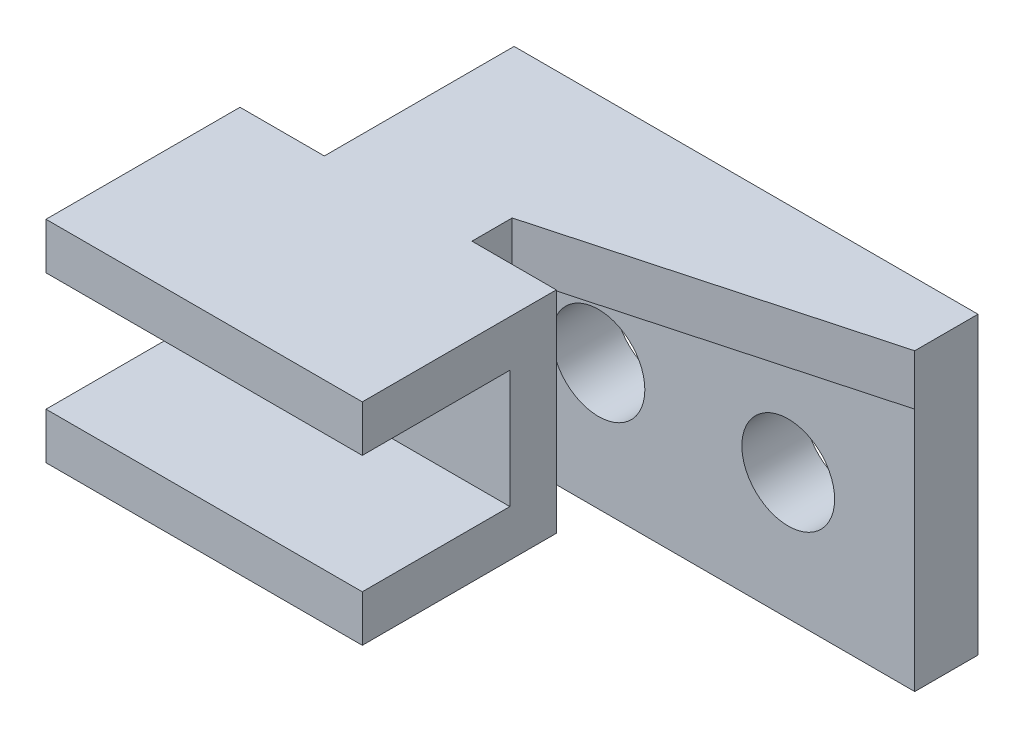
ISO-10303-21;
HEADER;
FILE_DESCRIPTION(('STEP AP214'),'2;1');
FILE_NAME('part.step','',(''),(''),'','','');
FILE_SCHEMA(('AUTOMOTIVE_DESIGN { 1 0 10303 214 1 1 1 1 }'));
ENDSEC;
DATA;
#1=APPLICATION_CONTEXT('core data for automotive mechanical design processes');
#2=APPLICATION_PROTOCOL_DEFINITION('international standard','automotive_design',2000,#1);
#3=PRODUCT_CONTEXT('',#1,'mechanical');
#4=PRODUCT('Part','Part','',(#3));
#5=PRODUCT_RELATED_PRODUCT_CATEGORY('part','',(#4));
#6=PRODUCT_DEFINITION_FORMATION('','',#4);
#7=PRODUCT_DEFINITION_CONTEXT('part definition',#1,'design');
#8=PRODUCT_DEFINITION('design','',#6,#7);
#9=PRODUCT_DEFINITION_SHAPE('','',#8);
#10=(LENGTH_UNIT() NAMED_UNIT(*) SI_UNIT(.MILLI.,.METRE.));
#11=(NAMED_UNIT(*) PLANE_ANGLE_UNIT() SI_UNIT($,.RADIAN.));
#12=(NAMED_UNIT(*) SI_UNIT($,.STERADIAN.) SOLID_ANGLE_UNIT());
#13=UNCERTAINTY_MEASURE_WITH_UNIT(LENGTH_MEASURE(1.E-05),#10,'distance_accuracy_value','');
#14=(GEOMETRIC_REPRESENTATION_CONTEXT(3) GLOBAL_UNCERTAINTY_ASSIGNED_CONTEXT((#13)) GLOBAL_UNIT_ASSIGNED_CONTEXT((#10,
#11,#12)) REPRESENTATION_CONTEXT('',''));
#15=CARTESIAN_POINT('',(0.,0.,0.));
#16=DIRECTION('',(0.,0.,1.));
#17=DIRECTION('',(1.,0.,0.));
#18=AXIS2_PLACEMENT_3D('',#15,#16,#17);
#19=CARTESIAN_POINT('',(0.,0.,15.));
#20=DIRECTION('',(0.,0.,1.));
#21=DIRECTION('',(1.,0.,0.));
#22=AXIS2_PLACEMENT_3D('',#19,#20,#21);
#23=PLANE('',#22);
#24=CARTESIAN_POINT('',(80.,30.,15.));
#25=DIRECTION('',(0.,0.,1.));
#26=DIRECTION('',(1.,0.,0.));
#27=AXIS2_PLACEMENT_3D('',#24,#25,#26);
#28=CIRCLE('',#27,11.);
#29=CARTESIAN_POINT('',(91.,30.,15.));
#30=VERTEX_POINT('',#29);
#31=EDGE_CURVE('E214',#30,#30,#28,.T.);
#32=ORIENTED_EDGE('',*,*,#31,.F.);
#33=EDGE_LOOP('',(#32));
#34=FACE_BOUND('',#33,.T.);
#35=CARTESIAN_POINT('',(35.,30.,15.));
#36=DIRECTION('',(0.,0.,1.));
#37=DIRECTION('',(1.,0.,0.));
#38=AXIS2_PLACEMENT_3D('',#35,#36,#37);
#39=CIRCLE('',#38,11.);
#40=CARTESIAN_POINT('',(46.,30.,15.));
#41=VERTEX_POINT('',#40);
#42=EDGE_CURVE('E201',#41,#41,#39,.T.);
#43=ORIENTED_EDGE('',*,*,#42,.F.);
#44=EDGE_LOOP('',(#43));
#45=FACE_BOUND('',#44,.T.);
#46=DIRECTION('',(0.,-1.,0.));
#47=VECTOR('',#46,1.);
#48=CARTESIAN_POINT('',(12.,0.,15.));
#49=LINE('',#48,#47);
#50=CARTESIAN_POINT('',(12.,58.,15.));
#51=VERTEX_POINT('',#50);
#52=CARTESIAN_POINT('',(12.,0.,15.));
#53=VERTEX_POINT('',#52);
#54=EDGE_CURVE('E267',#51,#53,#49,.T.);
#55=ORIENTED_EDGE('',*,*,#54,.T.);
#56=DIRECTION('',(1.,0.,0.));
#57=VECTOR('',#56,1.);
#58=CARTESIAN_POINT('',(0.,0.,15.));
#59=LINE('',#58,#57);
#60=CARTESIAN_POINT('',(110.,0.,15.));
#61=VERTEX_POINT('',#60);
#62=EDGE_CURVE('E291',#53,#61,#59,.T.);
#63=ORIENTED_EDGE('',*,*,#62,.T.);
#64=DIRECTION('',(0.,1.,0.));
#65=VECTOR('',#64,1.);
#66=CARTESIAN_POINT('',(110.,0.,15.));
#67=LINE('',#66,#65);
#68=CARTESIAN_POINT('',(110.,58.,15.));
#69=VERTEX_POINT('',#68);
#70=EDGE_CURVE('E292',#61,#69,#67,.T.);
#71=ORIENTED_EDGE('',*,*,#70,.T.);
#72=DIRECTION('',(-1.,0.,0.));
#73=VECTOR('',#72,1.);
#74=CARTESIAN_POINT('',(110.,58.,15.));
#75=LINE('',#74,#73);
#76=EDGE_CURVE('E278',#69,#51,#75,.T.);
#77=ORIENTED_EDGE('',*,*,#76,.T.);
#78=EDGE_LOOP('',(#55,#63,#71,#77));
#79=FACE_BOUND('',#78,.T.);
#80=ADVANCED_FACE('F44',(#34,#45,#79),#23,.T.);
#81=CARTESIAN_POINT('',(0.,70.,15.));
#82=DIRECTION('',(1.,0.,0.));
#83=DIRECTION('',(0.,0.,-1.));
#84=AXIS2_PLACEMENT_3D('',#81,#82,#83);
#85=PLANE('',#84);
#86=DIRECTION('',(0.,0.,-1.));
#87=VECTOR('',#86,1.);
#88=CARTESIAN_POINT('',(0.,0.,15.));
#89=LINE('',#88,#87);
#90=CARTESIAN_POINT('',(0.,0.,15.));
#91=VERTEX_POINT('',#90);
#92=CARTESIAN_POINT('',(0.,0.,0.));
#93=VERTEX_POINT('',#92);
#94=EDGE_CURVE('E52',#91,#93,#89,.T.);
#95=ORIENTED_EDGE('',*,*,#94,.F.);
#96=DIRECTION('',(0.,0.554700196225229,0.832050294337843));
#97=VECTOR('',#96,1.);
#98=CARTESIAN_POINT('',(0.,20.,45.));
#99=LINE('',#98,#97);
#100=CARTESIAN_POINT('',(0.,20.,45.));
#101=VERTEX_POINT('',#100);
#102=EDGE_CURVE('E264',#91,#101,#99,.T.);
#103=ORIENTED_EDGE('',*,*,#102,.T.);
#104=DIRECTION('',(0.,1.,0.));
#105=VECTOR('',#104,1.);
#106=CARTESIAN_POINT('',(0.,58.,45.));
#107=LINE('',#106,#105);
#108=CARTESIAN_POINT('',(0.,70.,45.));
#109=VERTEX_POINT('',#108);
#110=EDGE_CURVE('E284',#101,#109,#107,.T.);
#111=ORIENTED_EDGE('',*,*,#110,.T.);
#112=DIRECTION('',(0.,0.,-1.));
#113=VECTOR('',#112,1.);
#114=CARTESIAN_POINT('',(0.,70.,15.));
#115=LINE('',#114,#113);
#116=CARTESIAN_POINT('',(0.,70.,0.));
#117=VERTEX_POINT('',#116);
#118=EDGE_CURVE('E298',#109,#117,#115,.T.);
#119=ORIENTED_EDGE('',*,*,#118,.T.);
#120=DIRECTION('',(0.,-1.,0.));
#121=VECTOR('',#120,1.);
#122=CARTESIAN_POINT('',(0.,70.,0.));
#123=LINE('',#122,#121);
#124=EDGE_CURVE('E289',#117,#93,#123,.T.);
#125=ORIENTED_EDGE('',*,*,#124,.T.);
#126=EDGE_LOOP('',(#95,#103,#111,#119,#125));
#127=FACE_BOUND('',#126,.T.);
#128=ADVANCED_FACE('F50',(#127),#85,.F.);
#129=CARTESIAN_POINT('',(0.,0.,15.));
#130=DIRECTION('',(0.,1.,0.));
#131=DIRECTION('',(0.,0.,1.));
#132=AXIS2_PLACEMENT_3D('',#129,#130,#131);
#133=PLANE('',#132);
#134=DIRECTION('',(1.,0.,0.));
#135=VECTOR('',#134,1.);
#136=CARTESIAN_POINT('',(0.,0.,0.));
#137=LINE('',#136,#135);
#138=CARTESIAN_POINT('',(110.,0.,0.));
#139=VERTEX_POINT('',#138);
#140=EDGE_CURVE('E299',#93,#139,#137,.T.);
#141=ORIENTED_EDGE('',*,*,#140,.T.);
#142=DIRECTION('',(0.,0.,-1.));
#143=VECTOR('',#142,1.);
#144=CARTESIAN_POINT('',(110.,0.,15.));
#145=LINE('',#144,#143);
#146=EDGE_CURVE('E309',#61,#139,#145,.T.);
#147=ORIENTED_EDGE('',*,*,#146,.F.);
#148=ORIENTED_EDGE('',*,*,#62,.F.);
#149=EDGE_CURVE('E288',#91,#53,#59,.T.);
#150=ORIENTED_EDGE('',*,*,#149,.F.);
#151=ORIENTED_EDGE('',*,*,#94,.T.);
#152=EDGE_LOOP('',(#141,#147,#148,#150,#151));
#153=FACE_BOUND('',#152,.T.);
#154=ADVANCED_FACE('F317',(#153),#133,.F.);
#155=CARTESIAN_POINT('',(110.,0.,15.));
#156=DIRECTION('',(-1.,0.,0.));
#157=DIRECTION('',(0.,0.,1.));
#158=AXIS2_PLACEMENT_3D('',#155,#156,#157);
#159=PLANE('',#158);
#160=DIRECTION('',(0.,1.,0.));
#161=VECTOR('',#160,1.);
#162=CARTESIAN_POINT('',(110.,0.,0.));
#163=LINE('',#162,#161);
#164=CARTESIAN_POINT('',(110.,70.,0.));
#165=VERTEX_POINT('',#164);
#166=EDGE_CURVE('E301',#139,#165,#163,.T.);
#167=ORIENTED_EDGE('',*,*,#166,.T.);
#168=DIRECTION('',(0.,0.,-1.));
#169=VECTOR('',#168,1.);
#170=CARTESIAN_POINT('',(110.,70.,15.));
#171=LINE('',#170,#169);
#172=CARTESIAN_POINT('',(110.,70.,15.));
#173=VERTEX_POINT('',#172);
#174=EDGE_CURVE('E310',#173,#165,#171,.T.);
#175=ORIENTED_EDGE('',*,*,#174,.F.);
#176=DIRECTION('',(0.,1.,0.));
#177=VECTOR('',#176,1.);
#178=CARTESIAN_POINT('',(110.,58.,15.));
#179=LINE('',#178,#177);
#180=EDGE_CURVE('E287',#69,#173,#179,.T.);
#181=ORIENTED_EDGE('',*,*,#180,.F.);
#182=ORIENTED_EDGE('',*,*,#70,.F.);
#183=ORIENTED_EDGE('',*,*,#146,.T.);
#184=EDGE_LOOP('',(#167,#175,#181,#182,#183));
#185=FACE_BOUND('',#184,.T.);
#186=ADVANCED_FACE('F326',(#185),#159,.F.);
#187=CARTESIAN_POINT('',(110.,70.,15.));
#188=DIRECTION('',(0.,-1.,0.));
#189=DIRECTION('',(0.,0.,-1.));
#190=AXIS2_PLACEMENT_3D('',#187,#188,#189);
#191=PLANE('',#190);
#192=DIRECTION('',(-1.,0.,0.));
#193=VECTOR('',#192,1.);
#194=CARTESIAN_POINT('',(110.,70.,0.));
#195=LINE('',#194,#193);
#196=EDGE_CURVE('E303',#165,#117,#195,.T.);
#197=ORIENTED_EDGE('',*,*,#196,.T.);
#198=ORIENTED_EDGE('',*,*,#118,.F.);
#199=DIRECTION('',(-1.,0.,0.));
#200=VECTOR('',#199,1.);
#201=CARTESIAN_POINT('',(17.5,70.,45.));
#202=LINE('',#201,#200);
#203=CARTESIAN_POINT('',(-20.,70.,45.));
#204=VERTEX_POINT('',#203);
#205=EDGE_CURVE('E239',#109,#204,#202,.T.);
#206=ORIENTED_EDGE('',*,*,#205,.T.);
#207=DIRECTION('',(0.,0.,1.));
#208=VECTOR('',#207,1.);
#209=CARTESIAN_POINT('',(-20.,70.,56.));
#210=LINE('',#209,#208);
#211=CARTESIAN_POINT('',(-20.,70.,91.));
#212=VERTEX_POINT('',#211);
#213=EDGE_CURVE('E231',#204,#212,#210,.T.);
#214=ORIENTED_EDGE('',*,*,#213,.T.);
#215=DIRECTION('',(1.,0.,0.));
#216=VECTOR('',#215,1.);
#217=CARTESIAN_POINT('',(-20.,70.,91.));
#218=LINE('',#217,#216);
#219=CARTESIAN_POINT('',(55.,70.,91.));
#220=VERTEX_POINT('',#219);
#221=EDGE_CURVE('E196',#212,#220,#218,.T.);
#222=ORIENTED_EDGE('',*,*,#221,.T.);
#223=DIRECTION('',(0.,0.,-1.));
#224=VECTOR('',#223,1.);
#225=CARTESIAN_POINT('',(55.,70.,45.));
#226=LINE('',#225,#224);
#227=CARTESIAN_POINT('',(55.,70.,45.));
#228=VERTEX_POINT('',#227);
#229=EDGE_CURVE('E240',#220,#228,#226,.T.);
#230=ORIENTED_EDGE('',*,*,#229,.T.);
#231=CARTESIAN_POINT('',(35.,70.,45.));
#232=VERTEX_POINT('',#231);
#233=EDGE_CURVE('E241',#228,#232,#202,.T.);
#234=ORIENTED_EDGE('',*,*,#233,.T.);
#235=DIRECTION('',(0.,0.,-1.));
#236=VECTOR('',#235,1.);
#237=CARTESIAN_POINT('',(35.,70.,45.));
#238=LINE('',#237,#236);
#239=CARTESIAN_POINT('',(35.,70.,35.4545454545454));
#240=VERTEX_POINT('',#239);
#241=EDGE_CURVE('E250',#232,#240,#238,.T.);
#242=ORIENTED_EDGE('',*,*,#241,.T.);
#243=DIRECTION('',(0.964763821237732,0.,-0.263117405792109));
#244=VECTOR('',#243,1.);
#245=CARTESIAN_POINT('',(0.,70.,45.));
#246=LINE('',#245,#244);
#247=EDGE_CURVE('E58',#240,#173,#246,.T.);
#248=ORIENTED_EDGE('',*,*,#247,.T.);
#249=ORIENTED_EDGE('',*,*,#174,.T.);
#250=EDGE_LOOP('',(#197,#198,#206,#214,#222,#230,#234,#242,#248,#249));
#251=FACE_BOUND('',#250,.T.);
#252=ADVANCED_FACE('F335',(#251),#191,.F.);
#253=CARTESIAN_POINT('',(0.,0.,0.));
#254=DIRECTION('',(0.,0.,1.));
#255=DIRECTION('',(1.,0.,0.));
#256=AXIS2_PLACEMENT_3D('',#253,#254,#255);
#257=PLANE('',#256);
#258=CARTESIAN_POINT('',(80.,30.,0.));
#259=DIRECTION('',(0.,0.,1.));
#260=DIRECTION('',(1.,0.,0.));
#261=AXIS2_PLACEMENT_3D('',#258,#259,#260);
#262=CIRCLE('',#261,11.);
#263=CARTESIAN_POINT('',(91.,30.,0.));
#264=VERTEX_POINT('',#263);
#265=EDGE_CURVE('E210',#264,#264,#262,.T.);
#266=ORIENTED_EDGE('',*,*,#265,.T.);
#267=EDGE_LOOP('',(#266));
#268=FACE_BOUND('',#267,.T.);
#269=CARTESIAN_POINT('',(35.,30.,0.));
#270=DIRECTION('',(0.,0.,1.));
#271=DIRECTION('',(1.,0.,0.));
#272=AXIS2_PLACEMENT_3D('',#269,#270,#271);
#273=CIRCLE('',#272,11.);
#274=CARTESIAN_POINT('',(46.,30.,0.));
#275=VERTEX_POINT('',#274);
#276=EDGE_CURVE('E213',#275,#275,#273,.T.);
#277=ORIENTED_EDGE('',*,*,#276,.T.);
#278=EDGE_LOOP('',(#277));
#279=FACE_BOUND('',#278,.T.);
#280=ORIENTED_EDGE('',*,*,#124,.F.);
#281=ORIENTED_EDGE('',*,*,#196,.F.);
#282=ORIENTED_EDGE('',*,*,#166,.F.);
#283=ORIENTED_EDGE('',*,*,#140,.F.);
#284=EDGE_LOOP('',(#280,#281,#282,#283));
#285=FACE_BOUND('',#284,.T.);
#286=ADVANCED_FACE('F323',(#268,#279,#285),#257,.F.);
#287=CARTESIAN_POINT('',(0.,58.,45.));
#288=DIRECTION('',(0.263117405792109,0.,0.964763821237732));
#289=DIRECTION('',(0.964763821237732,0.,-0.263117405792109));
#290=AXIS2_PLACEMENT_3D('',#287,#288,#289);
#291=PLANE('',#290);
#292=DIRECTION('',(0.,1.,0.));
#293=VECTOR('',#292,1.);
#294=CARTESIAN_POINT('',(35.,58.,35.4545454545454));
#295=LINE('',#294,#293);
#296=CARTESIAN_POINT('',(35.,58.,35.4545454545455));
#297=VERTEX_POINT('',#296);
#298=EDGE_CURVE('E63',#297,#240,#295,.T.);
#299=ORIENTED_EDGE('',*,*,#298,.F.);
#300=DIRECTION('',(0.964763821237732,0.,-0.263117405792109));
#301=VECTOR('',#300,1.);
#302=CARTESIAN_POINT('',(0.,58.,45.));
#303=LINE('',#302,#301);
#304=EDGE_CURVE('E285',#297,#69,#303,.T.);
#305=ORIENTED_EDGE('',*,*,#304,.T.);
#306=ORIENTED_EDGE('',*,*,#180,.T.);
#307=ORIENTED_EDGE('',*,*,#247,.F.);
#308=EDGE_LOOP('',(#299,#305,#306,#307));
#309=FACE_BOUND('',#308,.T.);
#310=ADVANCED_FACE('F331',(#309),#291,.T.);
#311=CARTESIAN_POINT('',(0.,58.,0.));
#312=DIRECTION('',(0.,1.,0.));
#313=DIRECTION('',(0.,0.,1.));
#314=AXIS2_PLACEMENT_3D('',#311,#312,#313);
#315=PLANE('',#314);
#316=ORIENTED_EDGE('',*,*,#304,.F.);
#317=DIRECTION('',(0.,0.,-1.));
#318=VECTOR('',#317,1.);
#319=CARTESIAN_POINT('',(35.,58.,45.));
#320=LINE('',#319,#318);
#321=CARTESIAN_POINT('',(35.,58.,45.));
#322=VERTEX_POINT('',#321);
#323=EDGE_CURVE('E256',#322,#297,#320,.T.);
#324=ORIENTED_EDGE('',*,*,#323,.F.);
#325=DIRECTION('',(1.,0.,0.));
#326=VECTOR('',#325,1.);
#327=CARTESIAN_POINT('',(0.,58.,45.));
#328=LINE('',#327,#326);
#329=CARTESIAN_POINT('',(12.,58.,45.));
#330=VERTEX_POINT('',#329);
#331=EDGE_CURVE('E253',#330,#322,#328,.T.);
#332=ORIENTED_EDGE('',*,*,#331,.F.);
#333=DIRECTION('',(0.,0.,-1.));
#334=VECTOR('',#333,1.);
#335=CARTESIAN_POINT('',(12.,58.,0.));
#336=LINE('',#335,#334);
#337=EDGE_CURVE('E11',#330,#51,#336,.T.);
#338=ORIENTED_EDGE('',*,*,#337,.T.);
#339=ORIENTED_EDGE('',*,*,#76,.F.);
#340=EDGE_LOOP('',(#316,#324,#332,#338,#339));
#341=FACE_BOUND('',#340,.T.);
#342=ADVANCED_FACE('F343',(#341),#315,.F.);
#343=CARTESIAN_POINT('',(12.,20.,45.));
#344=DIRECTION('',(0.,-0.832050294337843,0.554700196225229));
#345=DIRECTION('',(0.,-0.554700196225229,-0.832050294337844));
#346=AXIS2_PLACEMENT_3D('',#343,#344,#345);
#347=PLANE('',#346);
#348=ORIENTED_EDGE('',*,*,#102,.F.);
#349=ORIENTED_EDGE('',*,*,#149,.T.);
#350=DIRECTION('',(0.,0.554700196225229,0.832050294337843));
#351=VECTOR('',#350,1.);
#352=CARTESIAN_POINT('',(12.,20.,45.));
#353=LINE('',#352,#351);
#354=CARTESIAN_POINT('',(12.,20.,45.));
#355=VERTEX_POINT('',#354);
#356=EDGE_CURVE('E266',#53,#355,#353,.T.);
#357=ORIENTED_EDGE('',*,*,#356,.T.);
#358=DIRECTION('',(-1.,0.,0.));
#359=VECTOR('',#358,1.);
#360=CARTESIAN_POINT('',(12.,20.,45.));
#361=LINE('',#360,#359);
#362=EDGE_CURVE('E274',#355,#101,#361,.T.);
#363=ORIENTED_EDGE('',*,*,#362,.T.);
#364=EDGE_LOOP('',(#348,#349,#357,#363));
#365=FACE_BOUND('',#364,.T.);
#366=ADVANCED_FACE('F365',(#365),#347,.T.);
#367=CARTESIAN_POINT('',(12.,0.,0.));
#368=DIRECTION('',(1.,0.,0.));
#369=DIRECTION('',(0.,0.,-1.));
#370=AXIS2_PLACEMENT_3D('',#367,#368,#369);
#371=PLANE('',#370);
#372=ORIENTED_EDGE('',*,*,#337,.F.);
#373=DIRECTION('',(0.,1.,0.));
#374=VECTOR('',#373,1.);
#375=CARTESIAN_POINT('',(12.,58.,45.));
#376=LINE('',#375,#374);
#377=EDGE_CURVE('E275',#355,#330,#376,.T.);
#378=ORIENTED_EDGE('',*,*,#377,.F.);
#379=ORIENTED_EDGE('',*,*,#356,.F.);
#380=ORIENTED_EDGE('',*,*,#54,.F.);
#381=EDGE_LOOP('',(#372,#378,#379,#380));
#382=FACE_BOUND('',#381,.T.);
#383=ADVANCED_FACE('F338',(#382),#371,.T.);
#384=CARTESIAN_POINT('',(35.,58.,45.));
#385=DIRECTION('',(1.,0.,0.));
#386=DIRECTION('',(0.,0.,-1.));
#387=AXIS2_PLACEMENT_3D('',#384,#385,#386);
#388=PLANE('',#387);
#389=ORIENTED_EDGE('',*,*,#241,.F.);
#390=DIRECTION('',(0.,1.,0.));
#391=VECTOR('',#390,1.);
#392=CARTESIAN_POINT('',(35.,58.,45.));
#393=LINE('',#392,#391);
#394=EDGE_CURVE('E257',#322,#232,#393,.T.);
#395=ORIENTED_EDGE('',*,*,#394,.F.);
#396=ORIENTED_EDGE('',*,*,#323,.T.);
#397=ORIENTED_EDGE('',*,*,#298,.T.);
#398=EDGE_LOOP('',(#389,#395,#396,#397));
#399=FACE_BOUND('',#398,.T.);
#400=ADVANCED_FACE('F352',(#399),#388,.T.);
#401=CARTESIAN_POINT('',(17.5,59.,45.));
#402=DIRECTION('',(0.,0.,-1.));
#403=DIRECTION('',(-1.,0.,0.));
#404=AXIS2_PLACEMENT_3D('',#401,#402,#403);
#405=PLANE('',#404);
#406=ORIENTED_EDGE('',*,*,#205,.F.);
#407=ORIENTED_EDGE('',*,*,#110,.F.);
#408=DIRECTION('',(1.,0.,0.));
#409=VECTOR('',#408,1.);
#410=CARTESIAN_POINT('',(-20.,20.,45.));
#411=LINE('',#410,#409);
#412=CARTESIAN_POINT('',(-20.,20.,45.));
#413=VERTEX_POINT('',#412);
#414=EDGE_CURVE('E229',#413,#101,#411,.T.);
#415=ORIENTED_EDGE('',*,*,#414,.F.);
#416=DIRECTION('',(0.,1.,0.));
#417=VECTOR('',#416,1.);
#418=CARTESIAN_POINT('',(-20.,59.,45.));
#419=LINE('',#418,#417);
#420=EDGE_CURVE('E242',#413,#204,#419,.T.);
#421=ORIENTED_EDGE('',*,*,#420,.T.);
#422=EDGE_LOOP('',(#406,#407,#415,#421));
#423=FACE_BOUND('',#422,.T.);
#424=ADVANCED_FACE('F354',(#423),#405,.T.);
#425=DIRECTION('',(0.,1.,0.));
#426=VECTOR('',#425,1.);
#427=CARTESIAN_POINT('',(55.,59.,45.));
#428=LINE('',#427,#426);
#429=CARTESIAN_POINT('',(55.,20.,45.));
#430=VERTEX_POINT('',#429);
#431=EDGE_CURVE('E244',#430,#228,#428,.T.);
#432=ORIENTED_EDGE('',*,*,#431,.F.);
#433=EDGE_CURVE('E234',#355,#430,#411,.T.);
#434=ORIENTED_EDGE('',*,*,#433,.F.);
#435=ORIENTED_EDGE('',*,*,#377,.T.);
#436=ORIENTED_EDGE('',*,*,#331,.T.);
#437=ORIENTED_EDGE('',*,*,#394,.T.);
#438=ORIENTED_EDGE('',*,*,#233,.F.);
#439=EDGE_LOOP('',(#432,#434,#435,#436,#437,#438));
#440=FACE_BOUND('',#439,.T.);
#441=ADVANCED_FACE('F346',(#440),#405,.T.);
#442=CARTESIAN_POINT('',(55.,59.,45.));
#443=DIRECTION('',(1.,0.,0.));
#444=DIRECTION('',(0.,0.,-1.));
#445=AXIS2_PLACEMENT_3D('',#442,#443,#444);
#446=PLANE('',#445);
#447=ORIENTED_EDGE('',*,*,#229,.F.);
#448=DIRECTION('',(0.,-1.,0.));
#449=VECTOR('',#448,1.);
#450=CARTESIAN_POINT('',(55.,70.,91.));
#451=LINE('',#450,#449);
#452=CARTESIAN_POINT('',(55.,59.,91.));
#453=VERTEX_POINT('',#452);
#454=EDGE_CURVE('E195',#220,#453,#451,.T.);
#455=ORIENTED_EDGE('',*,*,#454,.T.);
#456=DIRECTION('',(0.,0.,-1.));
#457=VECTOR('',#456,1.);
#458=CARTESIAN_POINT('',(55.,59.,80.));
#459=LINE('',#458,#457);
#460=CARTESIAN_POINT('',(55.,59.,56.));
#461=VERTEX_POINT('',#460);
#462=EDGE_CURVE('E208',#453,#461,#459,.T.);
#463=ORIENTED_EDGE('',*,*,#462,.T.);
#464=DIRECTION('',(0.,1.,0.));
#465=VECTOR('',#464,1.);
#466=CARTESIAN_POINT('',(55.,59.,56.));
#467=LINE('',#466,#465);
#468=CARTESIAN_POINT('',(55.,31.,56.));
#469=VERTEX_POINT('',#468);
#470=EDGE_CURVE('E247',#469,#461,#467,.T.);
#471=ORIENTED_EDGE('',*,*,#470,.F.);
#472=DIRECTION('',(0.,0.,1.));
#473=VECTOR('',#472,1.);
#474=CARTESIAN_POINT('',(55.,31.,56.));
#475=LINE('',#474,#473);
#476=CARTESIAN_POINT('',(55.,31.,91.));
#477=VERTEX_POINT('',#476);
#478=EDGE_CURVE('E221',#469,#477,#475,.T.);
#479=ORIENTED_EDGE('',*,*,#478,.T.);
#480=DIRECTION('',(0.,-1.,0.));
#481=VECTOR('',#480,1.);
#482=CARTESIAN_POINT('',(55.,31.,91.));
#483=LINE('',#482,#481);
#484=CARTESIAN_POINT('',(55.,20.,91.));
#485=VERTEX_POINT('',#484);
#486=EDGE_CURVE('E182',#477,#485,#483,.T.);
#487=ORIENTED_EDGE('',*,*,#486,.T.);
#488=DIRECTION('',(0.,0.,-1.));
#489=VECTOR('',#488,1.);
#490=CARTESIAN_POINT('',(55.,20.,80.));
#491=LINE('',#490,#489);
#492=EDGE_CURVE('E174',#485,#430,#491,.T.);
#493=ORIENTED_EDGE('',*,*,#492,.T.);
#494=ORIENTED_EDGE('',*,*,#431,.T.);
#495=EDGE_LOOP('',(#447,#455,#463,#471,#479,#487,#493,#494));
#496=FACE_BOUND('',#495,.T.);
#497=ADVANCED_FACE('F462',(#496),#446,.T.);
#498=CARTESIAN_POINT('',(55.,59.,56.));
#499=DIRECTION('',(0.,0.,1.));
#500=DIRECTION('',(1.,0.,0.));
#501=AXIS2_PLACEMENT_3D('',#498,#499,#500);
#502=PLANE('',#501);
#503=DIRECTION('',(1.,0.,0.));
#504=VECTOR('',#503,1.);
#505=CARTESIAN_POINT('',(-20.,59.,56.));
#506=LINE('',#505,#504);
#507=CARTESIAN_POINT('',(-20.,59.,56.));
#508=VERTEX_POINT('',#507);
#509=EDGE_CURVE('E222',#508,#461,#506,.T.);
#510=ORIENTED_EDGE('',*,*,#509,.F.);
#511=DIRECTION('',(0.,1.,0.));
#512=VECTOR('',#511,1.);
#513=CARTESIAN_POINT('',(-20.,59.,56.));
#514=LINE('',#513,#512);
#515=CARTESIAN_POINT('',(-20.,31.,56.));
#516=VERTEX_POINT('',#515);
#517=EDGE_CURVE('E252',#516,#508,#514,.T.);
#518=ORIENTED_EDGE('',*,*,#517,.F.);
#519=DIRECTION('',(1.,0.,0.));
#520=VECTOR('',#519,1.);
#521=CARTESIAN_POINT('',(-20.,31.,56.));
#522=LINE('',#521,#520);
#523=EDGE_CURVE('E167',#516,#469,#522,.T.);
#524=ORIENTED_EDGE('',*,*,#523,.T.);
#525=ORIENTED_EDGE('',*,*,#470,.T.);
#526=EDGE_LOOP('',(#510,#518,#524,#525));
#527=FACE_BOUND('',#526,.T.);
#528=ADVANCED_FACE('F478',(#527),#502,.T.);
#529=CARTESIAN_POINT('',(-20.,59.,56.));
#530=DIRECTION('',(-1.,0.,0.));
#531=DIRECTION('',(0.,0.,1.));
#532=AXIS2_PLACEMENT_3D('',#529,#530,#531);
#533=PLANE('',#532);
#534=ORIENTED_EDGE('',*,*,#213,.F.);
#535=ORIENTED_EDGE('',*,*,#420,.F.);
#536=DIRECTION('',(0.,0.,-1.));
#537=VECTOR('',#536,1.);
#538=CARTESIAN_POINT('',(-20.,20.,80.));
#539=LINE('',#538,#537);
#540=CARTESIAN_POINT('',(-20.,20.,91.));
#541=VERTEX_POINT('',#540);
#542=EDGE_CURVE('E172',#541,#413,#539,.T.);
#543=ORIENTED_EDGE('',*,*,#542,.F.);
#544=DIRECTION('',(0.,-1.,0.));
#545=VECTOR('',#544,1.);
#546=CARTESIAN_POINT('',(-20.,31.,91.));
#547=LINE('',#546,#545);
#548=CARTESIAN_POINT('',(-20.,31.,91.));
#549=VERTEX_POINT('',#548);
#550=EDGE_CURVE('E181',#549,#541,#547,.T.);
#551=ORIENTED_EDGE('',*,*,#550,.F.);
#552=DIRECTION('',(0.,0.,1.));
#553=VECTOR('',#552,1.);
#554=CARTESIAN_POINT('',(-20.,31.,56.));
#555=LINE('',#554,#553);
#556=EDGE_CURVE('E161',#516,#549,#555,.T.);
#557=ORIENTED_EDGE('',*,*,#556,.F.);
#558=ORIENTED_EDGE('',*,*,#517,.T.);
#559=DIRECTION('',(0.,0.,-1.));
#560=VECTOR('',#559,1.);
#561=CARTESIAN_POINT('',(-20.,59.,80.));
#562=LINE('',#561,#560);
#563=CARTESIAN_POINT('',(-20.,59.,91.));
#564=VERTEX_POINT('',#563);
#565=EDGE_CURVE('E219',#564,#508,#562,.T.);
#566=ORIENTED_EDGE('',*,*,#565,.F.);
#567=DIRECTION('',(0.,-1.,0.));
#568=VECTOR('',#567,1.);
#569=CARTESIAN_POINT('',(-20.,70.,91.));
#570=LINE('',#569,#568);
#571=EDGE_CURVE('E192',#212,#564,#570,.T.);
#572=ORIENTED_EDGE('',*,*,#571,.F.);
#573=EDGE_LOOP('',(#534,#535,#543,#551,#557,#558,#566,#572));
#574=FACE_BOUND('',#573,.T.);
#575=ADVANCED_FACE('F190',(#574),#533,.T.);
#576=CARTESIAN_POINT('',(-20.,20.,80.));
#577=DIRECTION('',(0.,-1.,0.));
#578=DIRECTION('',(0.,0.,-1.));
#579=AXIS2_PLACEMENT_3D('',#576,#577,#578);
#580=PLANE('',#579);
#581=ORIENTED_EDGE('',*,*,#492,.F.);
#582=DIRECTION('',(1.,0.,0.));
#583=VECTOR('',#582,1.);
#584=CARTESIAN_POINT('',(-20.,20.,91.));
#585=LINE('',#584,#583);
#586=EDGE_CURVE('E183',#541,#485,#585,.T.);
#587=ORIENTED_EDGE('',*,*,#586,.F.);
#588=ORIENTED_EDGE('',*,*,#542,.T.);
#589=ORIENTED_EDGE('',*,*,#414,.T.);
#590=ORIENTED_EDGE('',*,*,#362,.F.);
#591=ORIENTED_EDGE('',*,*,#433,.T.);
#592=EDGE_LOOP('',(#581,#587,#588,#589,#590,#591));
#593=FACE_BOUND('',#592,.T.);
#594=ADVANCED_FACE('F500',(#593),#580,.T.);
#595=CARTESIAN_POINT('',(-20.,31.,56.));
#596=DIRECTION('',(0.,1.,0.));
#597=DIRECTION('',(0.,0.,1.));
#598=AXIS2_PLACEMENT_3D('',#595,#596,#597);
#599=PLANE('',#598);
#600=ORIENTED_EDGE('',*,*,#478,.F.);
#601=ORIENTED_EDGE('',*,*,#523,.F.);
#602=ORIENTED_EDGE('',*,*,#556,.T.);
#603=DIRECTION('',(1.,0.,0.));
#604=VECTOR('',#603,1.);
#605=CARTESIAN_POINT('',(-20.,31.,91.));
#606=LINE('',#605,#604);
#607=EDGE_CURVE('E170',#549,#477,#606,.T.);
#608=ORIENTED_EDGE('',*,*,#607,.T.);
#609=EDGE_LOOP('',(#600,#601,#602,#608));
#610=FACE_BOUND('',#609,.T.);
#611=ADVANCED_FACE('F168',(#610),#599,.T.);
#612=CARTESIAN_POINT('',(-20.,59.,80.));
#613=DIRECTION('',(0.,-1.,0.));
#614=DIRECTION('',(0.,0.,-1.));
#615=AXIS2_PLACEMENT_3D('',#612,#613,#614);
#616=PLANE('',#615);
#617=ORIENTED_EDGE('',*,*,#462,.F.);
#618=DIRECTION('',(1.,0.,0.));
#619=VECTOR('',#618,1.);
#620=CARTESIAN_POINT('',(-20.,59.,91.));
#621=LINE('',#620,#619);
#622=EDGE_CURVE('E202',#564,#453,#621,.T.);
#623=ORIENTED_EDGE('',*,*,#622,.F.);
#624=ORIENTED_EDGE('',*,*,#565,.T.);
#625=ORIENTED_EDGE('',*,*,#509,.T.);
#626=EDGE_LOOP('',(#617,#623,#624,#625));
#627=FACE_BOUND('',#626,.T.);
#628=ADVANCED_FACE('F524',(#627),#616,.T.);
#629=CARTESIAN_POINT('',(35.,30.,0.));
#630=DIRECTION('',(0.,0.,1.));
#631=DIRECTION('',(1.,0.,0.));
#632=AXIS2_PLACEMENT_3D('',#629,#630,#631);
#633=CYLINDRICAL_SURFACE('',#632,11.);
#634=ORIENTED_EDGE('',*,*,#276,.F.);
#635=EDGE_LOOP('',(#634));
#636=FACE_BOUND('',#635,.T.);
#637=ORIENTED_EDGE('',*,*,#42,.T.);
#638=EDGE_LOOP('',(#637));
#639=FACE_BOUND('',#638,.T.);
#640=ADVANCED_FACE('F556',(#636,#639),#633,.F.);
#641=CARTESIAN_POINT('',(80.,30.,0.));
#642=DIRECTION('',(0.,0.,1.));
#643=DIRECTION('',(1.,0.,0.));
#644=AXIS2_PLACEMENT_3D('',#641,#642,#643);
#645=CYLINDRICAL_SURFACE('',#644,11.);
#646=ORIENTED_EDGE('',*,*,#265,.F.);
#647=EDGE_LOOP('',(#646));
#648=FACE_BOUND('',#647,.T.);
#649=ORIENTED_EDGE('',*,*,#31,.T.);
#650=EDGE_LOOP('',(#649));
#651=FACE_BOUND('',#650,.T.);
#652=ADVANCED_FACE('F550',(#648,#651),#645,.F.);
#653=CARTESIAN_POINT('',(-20.,70.,91.));
#654=DIRECTION('',(0.,0.,1.));
#655=DIRECTION('',(1.,0.,0.));
#656=AXIS2_PLACEMENT_3D('',#653,#654,#655);
#657=PLANE('',#656);
#658=ORIENTED_EDGE('',*,*,#454,.F.);
#659=ORIENTED_EDGE('',*,*,#221,.F.);
#660=ORIENTED_EDGE('',*,*,#571,.T.);
#661=ORIENTED_EDGE('',*,*,#622,.T.);
#662=EDGE_LOOP('',(#658,#659,#660,#661));
#663=FACE_BOUND('',#662,.T.);
#664=ADVANCED_FACE('F540',(#663),#657,.T.);
#665=CARTESIAN_POINT('',(-20.,31.,91.));
#666=DIRECTION('',(0.,0.,1.));
#667=DIRECTION('',(1.,0.,0.));
#668=AXIS2_PLACEMENT_3D('',#665,#666,#667);
#669=PLANE('',#668);
#670=ORIENTED_EDGE('',*,*,#486,.F.);
#671=ORIENTED_EDGE('',*,*,#607,.F.);
#672=ORIENTED_EDGE('',*,*,#550,.T.);
#673=ORIENTED_EDGE('',*,*,#586,.T.);
#674=EDGE_LOOP('',(#670,#671,#672,#673));
#675=FACE_BOUND('',#674,.T.);
#676=ADVANCED_FACE('F177',(#675),#669,.T.);
#677=CLOSED_SHELL('',(#80,#128,#154,#186,#252,#286,#310,#342,#366,#383,#400,#424,#441,#497,#528,
#575,#594,#611,#628,#640,#652,#664,#676));
#678=MANIFOLD_SOLID_BREP('B2',#677);
#679=ADVANCED_BREP_SHAPE_REPRESENTATION('',(#18,#678),#14);
#680=SHAPE_DEFINITION_REPRESENTATION(#9,#679);
ENDSEC;
END-ISO-10303-21;
